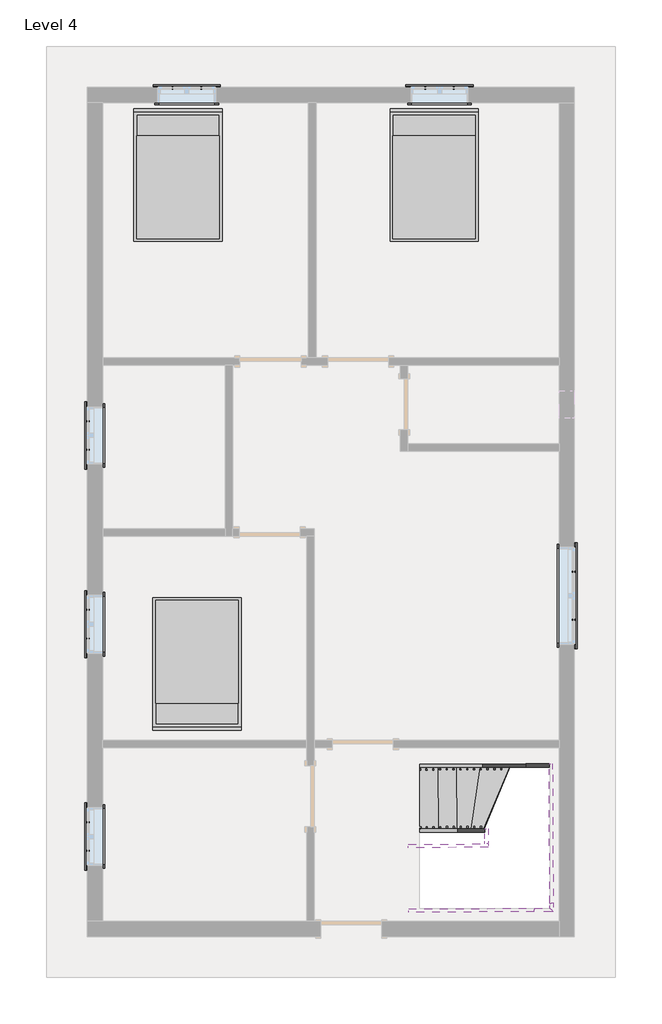
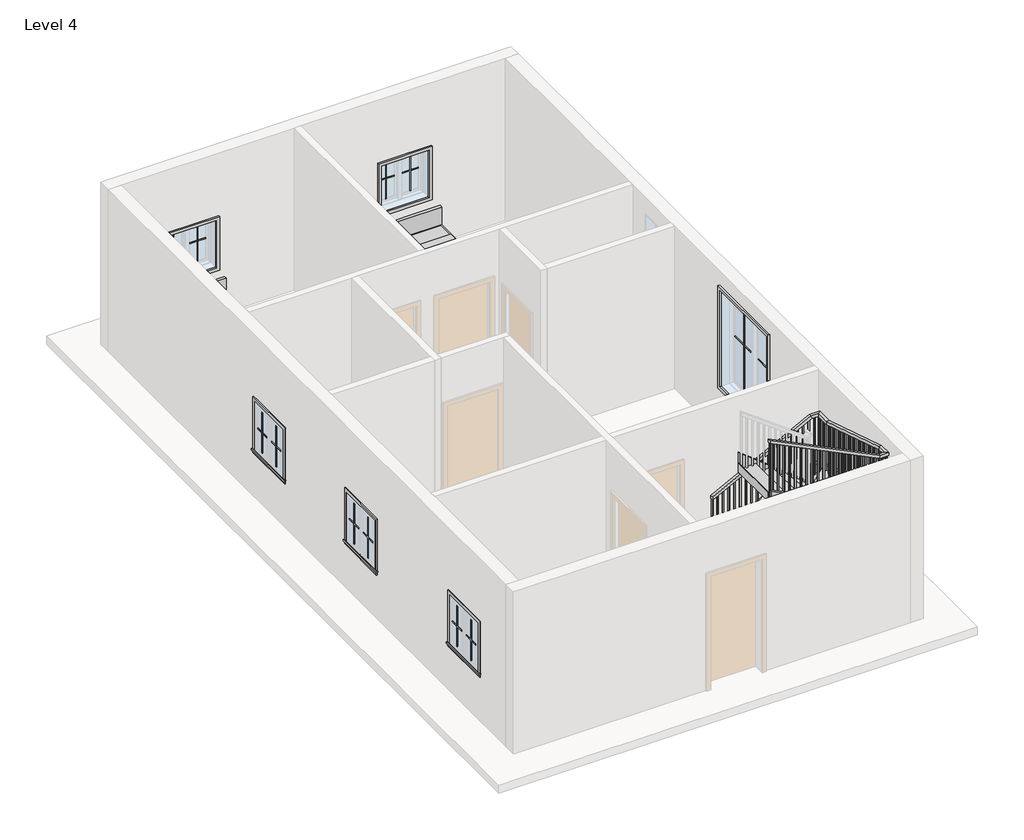
# One storey, part 2 of 2: 24 proxies, 9 members, 3 furniture elements, 1 railing, 1 stair flight.
"""IFC4 building model written with IfcOpenShell, lengths in millimetres."""

from ifc_helpers import new_model, si_unit, frame, origin, place, context, project, spatial, polyline, outline, extrude, faceted_brep, transform, mapped, element, save
from components import muntin_pattern_2x2_muntin_pattern_2x2_b3fe6957, muntin_pattern_2x2_muntin_pattern_2x2_3e0ecaf2, muntin_pattern_2x2_muntin_pattern_2x2_bff912c5, muntin_pattern_2x2_muntin_pattern_2x2_c2194282, trim_window_exterior_flat_with_sill_41619996, trim_window_exterior_flat_with_sill_e04b3088, trim_window_interior_flat_picture_frame_51c85655, trim_window_interior_flat_picture_frame_2a7685fe, bed_17739_bed_17739_15c61121, stair_flight_0f4fe1b0

model = new_model("IFC4")

# Units and contexts
model_context = context("Model", 3, world=origin())
ifc_project = project(units=[si_unit("LENGTHUNIT", "METRE", prefix="MILLI")], contexts=[model_context])

# Site, building, storey
site = spatial("IfcSite", under=ifc_project)
building = spatial("IfcBuilding", under=site)
storey = spatial("IfcBuildingStorey", under=building, Name="Level 4", Elevation=6400.8)

# Proxies
placement = place(None, origin())
muntin_pattern_2x2_muntin_pattern_2x2_shape = muntin_pattern_2x2_muntin_pattern_2x2_b3fe6957(model_context)
element("IfcBuildingElementProxy", 1, Name="Muntin Pattern_2x2 : Muntin Pattern_2x2", ObjectType="Muntin Pattern_2x2 : Muntin Pattern_2x2", at=placement, inside=storey, context=model_context, shape_type="MappedRepresentation", body=[
    mapped(muntin_pattern_2x2_muntin_pattern_2x2_shape, transform((-3622.2040084, 6872.3185985, 7385.05), x_axis=(1.0, 0.0, 0.0), y_axis=(0.0, 1.0, 0.0), z_axis=(0.0, 0.0, 1.0))),
])
element("IfcBuildingElementProxy", 2, Name="Muntin Pattern_2x2 : Muntin Pattern_2x2", ObjectType="Muntin Pattern_2x2 : Muntin Pattern_2x2", at=placement, inside=storey, context=model_context, shape_type="MappedRepresentation", body=[
    mapped(muntin_pattern_2x2_muntin_pattern_2x2_shape, transform((152.8709916, 6872.3185985, 7385.05), x_axis=(1.0, 0.0, 0.0), y_axis=(0.0, 1.0, 0.0), z_axis=(0.0, 0.0, 1.0))),
])
element("IfcBuildingElementProxy", 3, Name="Muntin Pattern_2x2 : Muntin Pattern_2x2", ObjectType="Muntin Pattern_2x2 : Muntin Pattern_2x2", at=placement, inside=storey, context=model_context, shape_type="MappedRepresentation", body=[
    mapped(muntin_pattern_2x2_muntin_pattern_2x2_shape, transform((-4884.2665084, 1466.8810985, 7385.05), x_axis=(0.0, 1.0, 0.0), y_axis=(-1.0, 0.0, 0.0), z_axis=(0.0, 0.0, 1.0))),
])
element("IfcBuildingElementProxy", 4, Name="Muntin Pattern_2x2 : Muntin Pattern_2x2", ObjectType="Muntin Pattern_2x2 : Muntin Pattern_2x2", at=placement, inside=storey, context=model_context, shape_type="MappedRepresentation", body=[
    mapped(muntin_pattern_2x2_muntin_pattern_2x2_shape, transform((-4884.2665084, -1352.5189015, 7385.05), x_axis=(0.0, 1.0, 0.0), y_axis=(-1.0, 0.0, 0.0), z_axis=(0.0, 0.0, 1.0))),
])
element("IfcBuildingElementProxy", 5, Name="Muntin Pattern_2x2 : Muntin Pattern_2x2", ObjectType="Muntin Pattern_2x2 : Muntin Pattern_2x2", at=placement, inside=storey, context=model_context, shape_type="MappedRepresentation", body=[
    mapped(muntin_pattern_2x2_muntin_pattern_2x2_shape, transform((-4884.2665084, -4524.3439015, 7385.05), x_axis=(0.0, 1.0, 0.0), y_axis=(-1.0, 0.0, 0.0), z_axis=(0.0, 0.0, 1.0))),
])
muntin_pattern_2x2_muntin_pattern_2x2_2_shape = muntin_pattern_2x2_muntin_pattern_2x2_3e0ecaf2(model_context)
element("IfcBuildingElementProxy", 6, Name="Muntin Pattern_2x2 : Muntin Pattern_2x2", ObjectType="Muntin Pattern_2x2 : Muntin Pattern_2x2", at=placement, inside=storey, context=model_context, shape_type="MappedRepresentation", body=[
    mapped(muntin_pattern_2x2_muntin_pattern_2x2_2_shape, transform((-3193.5790084, 6872.3185985, 7385.05), x_axis=(-1.0, 0.0, 0.0), y_axis=(0.0, -1.0, 0.0), z_axis=(0.0, 0.0, 1.0))),
])
element("IfcBuildingElementProxy", 7, Name="Muntin Pattern_2x2 : Muntin Pattern_2x2", ObjectType="Muntin Pattern_2x2 : Muntin Pattern_2x2", at=placement, inside=storey, context=model_context, shape_type="MappedRepresentation", body=[
    mapped(muntin_pattern_2x2_muntin_pattern_2x2_2_shape, transform((581.4959916, 6872.3185985, 7385.05), x_axis=(-1.0, 0.0, 0.0), y_axis=(0.0, -1.0, 0.0), z_axis=(0.0, 0.0, 1.0))),
])
element("IfcBuildingElementProxy", 8, Name="Muntin Pattern_2x2 : Muntin Pattern_2x2", ObjectType="Muntin Pattern_2x2 : Muntin Pattern_2x2", at=placement, inside=storey, context=model_context, shape_type="MappedRepresentation", body=[
    mapped(muntin_pattern_2x2_muntin_pattern_2x2_2_shape, transform((-4884.2665084, 1895.5060985, 7385.05), x_axis=(0.0, -1.0, 0.0), y_axis=(1.0, 0.0, 0.0), z_axis=(0.0, 0.0, 1.0))),
])
element("IfcBuildingElementProxy", 9, Name="Muntin Pattern_2x2 : Muntin Pattern_2x2", ObjectType="Muntin Pattern_2x2 : Muntin Pattern_2x2", at=placement, inside=storey, context=model_context, shape_type="MappedRepresentation", body=[
    mapped(muntin_pattern_2x2_muntin_pattern_2x2_2_shape, transform((-4884.2665084, -923.8939015, 7385.05), x_axis=(0.0, -1.0, 0.0), y_axis=(1.0, 0.0, 0.0), z_axis=(0.0, 0.0, 1.0))),
])
element("IfcBuildingElementProxy", 10, Name="Muntin Pattern_2x2 : Muntin Pattern_2x2", ObjectType="Muntin Pattern_2x2 : Muntin Pattern_2x2", at=placement, inside=storey, context=model_context, shape_type="MappedRepresentation", body=[
    mapped(muntin_pattern_2x2_muntin_pattern_2x2_2_shape, transform((-4884.2665084, -4095.7189015, 7385.05), x_axis=(0.0, -1.0, 0.0), y_axis=(1.0, 0.0, 0.0), z_axis=(0.0, 0.0, 1.0))),
])
muntin_pattern_2x2_muntin_pattern_2x2_3_shape = muntin_pattern_2x2_muntin_pattern_2x2_bff912c5(model_context)
element("IfcBuildingElementProxy", 11, Name="Muntin Pattern_2x2 : Muntin Pattern_2x2", ObjectType="Muntin Pattern_2x2 : Muntin Pattern_2x2", at=placement, inside=storey, context=model_context, shape_type="MappedRepresentation", body=[
    mapped(muntin_pattern_2x2_muntin_pattern_2x2_3_shape, transform((2373.7834916, -352.3939015, 7385.05), x_axis=(0.0, -1.0, 0.0), y_axis=(1.0, 0.0, 0.0), z_axis=(0.0, 0.0, 1.0))),
])
muntin_pattern_2x2_muntin_pattern_2x2_4_shape = muntin_pattern_2x2_muntin_pattern_2x2_c2194282(model_context)
element("IfcBuildingElementProxy", 12, Name="Muntin Pattern_2x2 : Muntin Pattern_2x2", ObjectType="Muntin Pattern_2x2 : Muntin Pattern_2x2", at=placement, inside=storey, context=model_context, shape_type="MappedRepresentation", body=[
    mapped(muntin_pattern_2x2_muntin_pattern_2x2_4_shape, transform((2373.7834916, -1073.1189015, 7385.05), x_axis=(0.0, 1.0, 0.0), y_axis=(-1.0, 0.0, 0.0), z_axis=(0.0, 0.0, 1.0))),
])
trim_window_exterior_flat_with_sill_shape = trim_window_exterior_flat_with_sill_41619996(model_context)
element("IfcBuildingElementProxy", 13, Name="Trim-Window-Exterior-Flat : with Sill", ObjectType="Trim-Window-Exterior-Flat : with Sill", at=placement, inside=storey, context=model_context, shape_type="MappedRepresentation", body=[
    mapped(trim_window_exterior_flat_with_sill_shape, transform((-3407.8915084, 6881.8435985, 8229.6), x_axis=(-1.0, 0.0, 0.0), y_axis=(0.0, 0.0, 1.0), z_axis=(0.0, 1.0, 0.0))),
])
element("IfcBuildingElementProxy", 14, Name="Trim-Window-Exterior-Flat : with Sill", ObjectType="Trim-Window-Exterior-Flat : with Sill", at=placement, inside=storey, context=model_context, shape_type="MappedRepresentation", body=[
    mapped(trim_window_exterior_flat_with_sill_shape, transform((367.1834916, 6881.8435985, 8229.6), x_axis=(-1.0, 0.0, 0.0), y_axis=(0.0, 0.0, 1.0), z_axis=(0.0, 1.0, 0.0))),
])
element("IfcBuildingElementProxy", 15, Name="Trim-Window-Exterior-Flat : with Sill", ObjectType="Trim-Window-Exterior-Flat : with Sill", at=placement, inside=storey, context=model_context, shape_type="MappedRepresentation", body=[
    mapped(trim_window_exterior_flat_with_sill_shape, transform((-4893.7915084, 1681.1935985, 8229.6), x_axis=(0.0, -1.0, 0.0), y_axis=(0.0, 0.0, 1.0), z_axis=(-1.0, 0.0, 0.0))),
])
element("IfcBuildingElementProxy", 16, Name="Trim-Window-Exterior-Flat : with Sill", ObjectType="Trim-Window-Exterior-Flat : with Sill", at=placement, inside=storey, context=model_context, shape_type="MappedRepresentation", body=[
    mapped(trim_window_exterior_flat_with_sill_shape, transform((-4893.7915084, -1138.2064015, 8229.6), x_axis=(0.0, -1.0, 0.0), y_axis=(0.0, 0.0, 1.0), z_axis=(-1.0, 0.0, 0.0))),
])
element("IfcBuildingElementProxy", 17, Name="Trim-Window-Exterior-Flat : with Sill", ObjectType="Trim-Window-Exterior-Flat : with Sill", at=placement, inside=storey, context=model_context, shape_type="MappedRepresentation", body=[
    mapped(trim_window_exterior_flat_with_sill_shape, transform((-4893.7915084, -4310.0314015, 8229.6), x_axis=(0.0, -1.0, 0.0), y_axis=(0.0, 0.0, 1.0), z_axis=(-1.0, 0.0, 0.0))),
])
trim_window_exterior_flat_with_sill_2_shape = trim_window_exterior_flat_with_sill_e04b3088(model_context)
element("IfcBuildingElementProxy", 18, Name="Trim-Window-Exterior-Flat : with Sill", ObjectType="Trim-Window-Exterior-Flat : with Sill", at=placement, inside=storey, context=model_context, shape_type="MappedRepresentation", body=[
    mapped(trim_window_exterior_flat_with_sill_2_shape, transform((2383.3084916, -712.7564015, 9144.0), x_axis=(0.0, 1.0, 0.0), y_axis=(0.0, 0.0, 1.0), z_axis=(1.0, 0.0, 0.0))),
])
trim_window_interior_flat_picture_frame_shape = trim_window_interior_flat_picture_frame_51c85655(model_context)
element("IfcBuildingElementProxy", 19, Name="Trim-Window-Interior-Flat : Picture Frame", ObjectType="Trim-Window-Interior-Flat : Picture Frame", at=placement, inside=storey, context=model_context, shape_type="MappedRepresentation", body=[
    mapped(trim_window_interior_flat_picture_frame_shape, transform((-3407.8915084, 6653.2435985, 8229.6), x_axis=(1.0, 0.0, 0.0), y_axis=(0.0, 0.0, 1.0), z_axis=(0.0, -1.0, 0.0))),
])
element("IfcBuildingElementProxy", 20, Name="Trim-Window-Interior-Flat : Picture Frame", ObjectType="Trim-Window-Interior-Flat : Picture Frame", at=placement, inside=storey, context=model_context, shape_type="MappedRepresentation", body=[
    mapped(trim_window_interior_flat_picture_frame_shape, transform((367.1834916, 6653.2435985, 8229.6), x_axis=(1.0, 0.0, 0.0), y_axis=(0.0, 0.0, 1.0), z_axis=(0.0, -1.0, 0.0))),
])
element("IfcBuildingElementProxy", 21, Name="Trim-Window-Interior-Flat : Picture Frame", ObjectType="Trim-Window-Interior-Flat : Picture Frame", at=placement, inside=storey, context=model_context, shape_type="MappedRepresentation", body=[
    mapped(trim_window_interior_flat_picture_frame_shape, transform((-4665.1915084, 1681.1935985, 8229.6), x_axis=(0.0, 1.0, 0.0), y_axis=(0.0, 0.0, 1.0), z_axis=(1.0, 0.0, 0.0))),
])
element("IfcBuildingElementProxy", 22, Name="Trim-Window-Interior-Flat : Picture Frame", ObjectType="Trim-Window-Interior-Flat : Picture Frame", at=placement, inside=storey, context=model_context, shape_type="MappedRepresentation", body=[
    mapped(trim_window_interior_flat_picture_frame_shape, transform((-4665.1915084, -1138.2064015, 8229.6), x_axis=(0.0, 1.0, 0.0), y_axis=(0.0, 0.0, 1.0), z_axis=(1.0, 0.0, 0.0))),
])
element("IfcBuildingElementProxy", 23, Name="Trim-Window-Interior-Flat : Picture Frame", ObjectType="Trim-Window-Interior-Flat : Picture Frame", at=placement, inside=storey, context=model_context, shape_type="MappedRepresentation", body=[
    mapped(trim_window_interior_flat_picture_frame_shape, transform((-4665.1915084, -4310.0314015, 8229.6), x_axis=(0.0, 1.0, 0.0), y_axis=(0.0, 0.0, 1.0), z_axis=(1.0, 0.0, 0.0))),
])
trim_window_interior_flat_picture_frame_2_shape = trim_window_interior_flat_picture_frame_2a7685fe(model_context)
element("IfcBuildingElementProxy", 24, Name="Trim-Window-Interior-Flat : Picture Frame", ObjectType="Trim-Window-Interior-Flat : Picture Frame", at=placement, inside=storey, context=model_context, shape_type="MappedRepresentation", body=[
    mapped(trim_window_interior_flat_picture_frame_2_shape, transform((2154.7084916, -712.7564015, 9144.0), x_axis=(0.0, -1.0, 0.0), y_axis=(0.0, 0.0, 1.0), z_axis=(-1.0, 0.0, 0.0))),
])

# Furniture
bed_17739_bed_17739_shape = bed_17739_bed_17739_15c61121(model_context)
element("IfcFurniture", 25, ObjectType="Bed_17739 : Bed_17739", at=placement, inside=storey, context=model_context, shape_type="MappedRepresentation", body=[
    mapped(bed_17739_bed_17739_shape, transform((-3541.2415084, 5548.3435985, 6400.8), x_axis=(1.0, 0.0, 0.0), y_axis=(0.0, 1.0, 0.0), z_axis=(0.0, 0.0, 1.0))),
])
element("IfcFurniture", 26, ObjectType="Bed_17739 : Bed_17739", at=placement, inside=storey, context=model_context, shape_type="MappedRepresentation", body=[
    mapped(bed_17739_bed_17739_shape, transform((287.8084916, 5548.3435985, 6400.8), x_axis=(1.0, 0.0, 0.0), y_axis=(0.0, 1.0, 0.0), z_axis=(0.0, 0.0, 1.0))),
])
element("IfcFurniture", 27, ObjectType="Bed_17739 : Bed_17739", at=placement, inside=storey, context=model_context, shape_type="MappedRepresentation", body=[
    mapped(bed_17739_bed_17739_shape, transform((-3255.4915084, -1709.7064015, 6400.8), x_axis=(-1.0, 0.0, 0.0), y_axis=(0.0, -1.0, 0.0), z_axis=(0.0, 0.0, 1.0))),
])

# Members
element("IfcMember", 28, ObjectType="Stringer - 2\" Width", at=placement, inside=storey, context=model_context, shape_type="SweptSolid", body=[
    extrude(outline(polyline([(149.3129896, -304.8), (0.0, 0.0), (1768.8429208, 0.0), (1918.1559104, -304.8000001), (149.3129896, -304.8)])), frame((68.8012135, -3282.7418259, 6804.1997735), z_axis=(-0.005162073969671357, 0.9999866764074068, 0.0), x_axis=(0.8980237466183221, 0.0046357267711000134, 0.43992256198892044)), (0.0, 0.0, 1.0), 50.8),
])
element("IfcMember", 29, ObjectType="Stringer - 2\" Width", at=placement, inside=storey, context=model_context, shape_type="SweptSolid", body=[
    extrude(outline(polyline([(1657.2641604, -3274.5419534), (1657.0019271, -3223.7426303), (2003.5241973, -3221.9538329), (2003.7864306, -3272.753156), (1657.2641604, -3274.5419534)])), frame((0.0, 0.0, 7582.353683), z_axis=(0.0, 0.0, 1.0), x_axis=(1.0, 0.0, 0.0)), (0.0, 0.0, 1.0), 339.4074379),
])
element("IfcMember", 30, ObjectType="Stringer - 2\" Width", at=placement, inside=storey, context=model_context, shape_type="SweptSolid", body=[
    extrude(outline(polyline([(47.2049979, -324.2228076), (-38.2916769, -48.0839082), (117.0107078, 0.0), (2125.7436964, 0.0), (2226.1278582, -324.2228076), (47.2049979, -324.2228076)])), frame((2003.7864306, -3272.753156, 7582.353683), z_axis=(0.9999866764074068, 0.005162073969671768, 0.0), x_axis=(0.004931129753271623, -0.9552486233011703, 0.2957629991066754)), (0.0, 0.0, 1.0), 50.8),
])
element("IfcMember", 31, ObjectType="Stringer - 2\" Width", at=placement, inside=storey, context=model_context, shape_type="SweptSolid", body=[
    extrude(outline(polyline([(2014.2687486, -5303.3668955), (2065.0680718, -5303.1046621), (2065.7306715, -5431.462157), (2014.669115, -5380.9250672), (2014.2687486, -5303.3668955)])), frame((0.0, 0.0, 8221.0291102), z_axis=(0.0, 0.0, 1.0), x_axis=(1.0, 0.0, 0.0)), (0.0, 0.0, 1.0), 319.0749838),
])
element("IfcMember", 32, ObjectType="Stringer - 2\" Width", at=placement, inside=storey, context=model_context, shape_type="SweptSolid", body=[
    extrude(outline(polyline([(2014.669115, -5380.9250672), (2065.7306715, -5431.462157), (1782.4368375, -5432.9245602), (1782.1746041, -5382.1252371), (2014.669115, -5380.9250672)])), frame((0.0, 0.0, 8221.0291102), z_axis=(0.0, 0.0, 1.0), x_axis=(1.0, 0.0, 0.0)), (0.0, 0.0, 1.0), 319.0749838),
])
element("IfcMember", 33, ObjectType="Stringer - 2\" Width", at=placement, inside=storey, context=model_context, shape_type="SweptSolid", body=[
    extrude(outline(polyline([(286.8047106, -304.8), (0.0, 0.0), (1331.6484515, 0.0), (1618.4531621, -304.8), (286.8047106, -304.8)])), frame((73.7836473, -4247.928966, 6647.3616111), z_axis=(-0.005162073969671482, 0.9999866764074068, 0.0), x_axis=(0.7282688430294204, 0.0037594277266083504, 0.6852812261953175)), (0.0, 0.0, 1.0), 50.8),
])
element("IfcMember", 34, ObjectType="Stringer - 2\" Width", at=placement, inside=storey, context=model_context, shape_type="SweptSolid", body=[
    extrude(outline(polyline([(660.780085, -304.8), (110.7389009, -51.080863), (134.3011229, 0.0), (545.7678218, 0.0), (1125.9670058, -267.6302075), (1108.8215849, -304.8), (660.780085, -304.8)])), frame((1043.319491, -4192.1234067, 7485.7637993), z_axis=(0.9999866764074068, 0.005162073969671282, 0.0), x_axis=(0.002162183372020065, -0.4188538515087163, 0.90805108669027)), (0.0, 0.0, 1.0), 50.8),
])
element("IfcMember", 35, ObjectType="Stringer - 2\" Width", at=placement, inside=storey, context=model_context, shape_type="SweptSolid", body=[
    extrude(outline(polyline([(-239.6623642, -304.8), (0.0, 0.0), (1521.9461582, 0.0), (1282.2837939, -304.8), (-239.6623642, -304.8)])), frame((1095.5610976, -4471.2574507, 8620.2987993), z_axis=(-0.005162073969672184, 0.9999866764074068, 0.0), x_axis=(-0.7860864868637559, -0.0040578906574323574, 0.6181032023000775)), (0.0, 0.0, 1.0), 50.8),
])
element("IfcMember", 36, ObjectType="Stringer - 2\" Width", at=placement, inside=storey, context=model_context, shape_type="SweptSolid", body=[
    extrude(outline(polyline([(-137.2719745, -288.0368905), (0.0, 0.0), (2080.7002403, 0.0), (1943.4282658, -288.0368905), (-137.2719745, -288.0368905)])), frame((1782.4368375, -5432.9245602, 8540.104094), z_axis=(-0.005162073969672376, 0.9999866764074068, 0.0), x_axis=(-0.9027127399072911, -0.004659932023802854, 0.43021854242071556)), (0.0, 0.0, 1.0), 50.8),
])

# Railing
element("IfcRailing", 37, ObjectType="Handrail - Rectangular", at=placement, inside=storey, context=model_context, shape_type="SolidModel", body=[
    faceted_brep([(68.8012135, -3282.7418259, 7992.5333333), (68.8012135, -3282.7418259, 7935.4032367), (69.0634468, -3333.5411491, 7935.4032367), (69.0634468, -3333.5411491, 7992.5333333), (1818.9474855, -3273.707321, 8893.0523232), (1831.2499413, -3273.643814, 8842.2523232), (1831.5121746, -3324.4431372, 8842.2523232), (1819.2097188, -3324.5066442, 8893.0523232), (2003.7864306, -3272.753156, 8893.0523232), (2003.7864306, -3272.753156, 8842.2523232), (1953.2493408, -3323.8147125, 8842.2523232), (1953.2493408, -3323.8147125, 8893.0523232), (2005.285328, -3563.1165554, 8893.0523232), (2005.3249947, -3570.8007251, 8842.2523232), (1954.5256716, -3571.0629585, 8842.2523232), (1954.4860048, -3563.3787887, 8893.0523232), (2013.5123671, -5156.842168, 9386.4998462), (2013.5520339, -5164.5263378, 9335.6998462), (1962.7527107, -5164.7885712, 9335.6998462), (1962.7130439, -5157.1044014, 9386.4998462), (2014.669115, -5380.9250672, 9386.4998462), (2014.669115, -5380.9250672, 9335.6998462), (1963.6075585, -5330.3879774, 9335.6998462), (1963.6075585, -5330.3879774, 9386.4998462), (1865.7077622, -5381.694027, 9386.4998462), (1853.7618085, -5381.7556937, 9335.6998462), (1853.4995752, -5330.9563705, 9335.6998462), (1865.4455288, -5330.8947038, 9386.4998462), (-96.1000106, -5391.8211588, 10363.2), (-96.362244, -5341.0218356, 10363.2), (-96.362244, -5341.0218356, 10306.4526208), (-96.1000106, -5391.8211588, 10306.4526208)], [[[0, 1, 2, 3]], [[1, 0, 4, 5]], [[2, 1, 5, 6]], [[3, 2, 6, 7]], [[0, 3, 7, 4]], [[5, 4, 8, 9]], [[6, 5, 9, 10]], [[7, 6, 10, 11]], [[4, 7, 11, 8]], [[9, 8, 12, 13]], [[10, 9, 13, 14]], [[11, 10, 14, 15]], [[8, 11, 15, 12]], [[13, 12, 16, 17]], [[14, 13, 17, 18]], [[15, 14, 18, 19]], [[12, 15, 19, 16]], [[17, 16, 20, 21]], [[18, 17, 21, 22]], [[19, 18, 22, 23]], [[16, 19, 23, 20]], [[21, 20, 24, 25]], [[22, 21, 25, 26]], [[23, 22, 26, 27]], [[20, 23, 27, 24]], [[28, 29, 30, 31]], [[25, 24, 28, 31]], [[26, 25, 31, 30]], [[27, 26, 30, 29]], [[24, 27, 29, 28]]]),
    extrude(outline(polyline([(223.8579732, 19.05), (1229.0021026, 19.05), (1229.0021026, 0.0), (233.3420268, 0.0), (223.8579732, 19.05)])), frame((-33.2605479, -5375.621561, 10508.4687693), z_axis=(-0.005162073969671937, 0.9999866764074068, 0.0), x_axis=(0.0, 0.0, -1.0)), (0.0, 0.0, 1.0), 19.05),
    extrude(outline(polyline([(223.8579732, 19.0499999), (1178.4204835, 19.0499999), (1178.4204835, 0.0), (233.3420268, 0.0), (223.8579732, 19.0499999)])), frame((68.3380984, -5375.0970942, 10457.8871502), z_axis=(-0.005162073969671937, 0.9999866764074068, 0.0), x_axis=(0.0, 0.0, -1.0)), (0.0, 0.0, 1.0), 19.05),
    extrude(outline(polyline([(223.8579732, 19.05), (1127.8388644, 19.05), (1127.8388644, 0.0), (233.3420268, 0.0), (223.8579732, 19.05)])), frame((169.9367448, -5374.5726275, 10407.3055311), z_axis=(-0.005162073969671937, 0.9999866764074068, 0.0), x_axis=(0.0, 0.0, -1.0)), (0.0, 0.0, 1.0), 19.05),
    extrude(outline(polyline([(223.8579732, 19.05), (1246.5905787, 19.05), (1246.5905787, 0.0), (233.3420268, 0.0), (223.8579732, 19.05)])), frame((271.5353911, -5374.0481608, 10356.723912), z_axis=(-0.005162073969671937, 0.9999866764074068, 0.0), x_axis=(0.0, 0.0, -1.0)), (0.0, 0.0, 1.0), 19.05),
    extrude(outline(polyline([(223.8579732, 19.05), (1196.0089596, 19.05), (1196.0089596, 0.0), (233.3420267, 0.0), (223.8579732, 19.05)])), frame((373.1340374, -5373.5236941, 10306.1422929), z_axis=(-0.005162073969671937, 0.9999866764074068, 0.0), x_axis=(0.0, 0.0, -1.0)), (0.0, 0.0, 1.0), 19.05),
    extrude(outline(polyline([(223.8579732, 19.05), (1314.7606738, 19.05), (1314.7606738, 0.0), (233.3420267, 0.0), (223.8579732, 19.05)])), frame((474.7326837, -5372.9992274, 10255.5606738), z_axis=(-0.005162073969671937, 0.9999866764074068, 0.0), x_axis=(0.0, 0.0, -1.0)), (0.0, 0.0, 1.0), 19.05),
    extrude(outline(polyline([(223.8579733, 19.05), (1264.1790548, 19.05), (1264.1790548, 0.0), (233.3420268, 0.0), (223.8579733, 19.05)])), frame((576.3313301, -5372.4747607, 10204.9790548), z_axis=(-0.005162073969671937, 0.9999866764074068, 0.0), x_axis=(0.0, 0.0, -1.0)), (0.0, 0.0, 1.0), 19.05),
    extrude(outline(polyline([(223.8579732, 19.05), (1213.5974357, 19.05), (1213.5974357, 0.0), (233.3420268, 0.0), (223.8579732, 19.05)])), frame((677.9299764, -5371.950294, 10154.3974357), z_axis=(-0.005162073969671937, 0.9999866764074068, 0.0), x_axis=(0.0, 0.0, -1.0)), (0.0, 0.0, 1.0), 19.05),
    extrude(outline(polyline([(223.8579732, 19.05), (1163.0158166, 19.05), (1163.0158166, 0.0), (233.3420268, 0.0), (223.8579732, 19.05)])), frame((779.5286227, -5371.4258272, 10103.8158166), z_axis=(-0.005162073969671937, 0.9999866764074068, 0.0), x_axis=(0.0, 0.0, -1.0)), (0.0, 0.0, 1.0), 19.05),
    extrude(outline(polyline([(223.8579732, 19.05), (1281.7675308, 19.05), (1281.7675308, 0.0), (233.3420268, 0.0), (223.8579732, 19.05)])), frame((881.127269, -5370.9013605, 10053.2341975), z_axis=(-0.005162073969671937, 0.9999866764074068, 0.0), x_axis=(0.0, 0.0, -1.0)), (0.0, 0.0, 1.0), 19.05),
    extrude(outline(polyline([(223.8579732, 19.0499999), (1231.1859117, 19.0499999), (1231.1859117, 0.0), (233.3420268, 0.0), (223.8579732, 19.0499999)])), frame((982.7259153, -5370.3768938, 10002.6525784), z_axis=(-0.005162073969671937, 0.9999866764074068, 0.0), x_axis=(0.0, 0.0, -1.0)), (0.0, 0.0, 1.0), 19.05),
    extrude(outline(polyline([(223.8579732, 19.05), (1180.6042926, 19.05), (1180.6042926, 0.0), (233.3420268, 0.0), (223.8579732, 19.05)])), frame((1084.3245617, -5369.8524271, 9952.0709593), z_axis=(-0.005162073969671937, 0.9999866764074068, 0.0), x_axis=(0.0, 0.0, -1.0)), (0.0, 0.0, 1.0), 19.05),
    extrude(outline(polyline([(223.8579732, 19.05), (1299.3560069, 19.05), (1299.3560069, 0.0), (233.3420268, 0.0), (223.8579732, 19.05)])), frame((1185.923208, -5369.3279604, 9901.4893402), z_axis=(-0.005162073969671937, 0.9999866764074068, 0.0), x_axis=(0.0, 0.0, -1.0)), (0.0, 0.0, 1.0), 19.05),
    extrude(outline(polyline([(223.8579732, 19.05), (1248.7743878, 19.05), (1248.7743878, 0.0), (233.3420268, 0.0), (223.8579732, 19.05)])), frame((1287.5218543, -5368.8034937, 9850.9077211), z_axis=(-0.005162073969671937, 0.9999866764074068, 0.0), x_axis=(0.0, 0.0, -1.0)), (0.0, 0.0, 1.0), 19.05),
    extrude(outline(polyline([(223.8579732, 19.0499999), (1198.1927687, 19.0499999), (1198.1927687, 0.0), (233.3420268, 0.0), (223.8579732, 19.0499999)])), frame((1389.1205006, -5368.2790269, 9800.326102), z_axis=(-0.005162073969671937, 0.9999866764074068, 0.0), x_axis=(0.0, 0.0, -1.0)), (0.0, 0.0, 1.0), 19.05),
    extrude(outline(polyline([(223.8579732, 19.05), (1147.6111496, 19.05), (1147.6111496, 0.0), (233.3420268, 0.0), (223.8579732, 19.05)])), frame((1490.719147, -5367.7545602, 9749.7444829), z_axis=(-0.005162073969671937, 0.9999866764074068, 0.0), x_axis=(0.0, 0.0, -1.0)), (0.0, 0.0, 1.0), 19.05),
    extrude(outline(polyline([(223.8579732, 19.05), (1097.0295305, 19.05), (1097.0295305, 0.0), (233.3420267, 0.0), (223.8579732, 19.05)])), frame((1592.3177933, -5367.2300935, 9699.1628638), z_axis=(-0.005162073969671937, 0.9999866764074068, 0.0), x_axis=(0.0, 0.0, -1.0)), (0.0, 0.0, 1.0), 19.05),
    extrude(outline(polyline([(223.8579733, 19.05), (1215.7812448, 19.05), (1215.7812448, 0.0), (233.3420268, 0.0), (223.8579733, 19.05)])), frame((1693.9164396, -5366.7056268, 9648.5812448), z_axis=(-0.005162073969671937, 0.9999866764074068, 0.0), x_axis=(0.0, 0.0, -1.0)), (0.0, 0.0, 1.0), 19.05),
    extrude(outline(polyline([(223.8579733, 19.05), (1165.1996257, 19.05), (1165.1996257, 0.0), (233.3420268, 0.0), (223.8579733, 19.05)])), frame((1795.5150859, -5366.1811601, 9597.9996257), z_axis=(-0.005162073969671937, 0.9999866764074068, 0.0), x_axis=(0.0, 0.0, -1.0)), (0.0, 0.0, 1.0), 19.05),
    extrude(outline(polyline([(1897.1137323, -5365.6566934), (1878.0639861, -5365.7550309), (1877.9656486, -5346.7052847), (1897.0153947, -5346.6069472), (1897.1137323, -5365.6566934)])), frame((0.0, 0.0, 8432.8), z_axis=(0.0, 0.0, 1.0), x_axis=(1.0, 0.0, 0.0)), (0.0, 0.0, 1.0), 902.8998462),
    extrude(outline(polyline([(1998.4829244, -5320.6828189), (1998.5812619, -5339.7325651), (1979.5315157, -5339.8309026), (1979.4331782, -5320.7811564), (1998.4829244, -5320.6828189)])), frame((0.0, 0.0, 8432.8), z_axis=(0.0, 0.0, 1.0), x_axis=(1.0, 0.0, 0.0)), (0.0, 0.0, 1.0), 902.8998462),
    extrude(outline(polyline([(1997.9584577, -5219.0841726), (1998.0567952, -5238.1339187), (1979.007049, -5238.2322563), (1978.9087115, -5219.1825101), (1997.9584577, -5219.0841726)])), frame((0.0, 0.0, 8432.8), z_axis=(0.0, 0.0, 1.0), x_axis=(1.0, 0.0, 0.0)), (0.0, 0.0, 1.0), 902.8998462),
    extrude(outline(polyline([(231.5490805, 19.05), (1119.8588311, 19.05), (1119.8588311, 0.0), (225.6509196, 0.0), (231.5490805, 19.05)])), frame((1978.4825823, -5136.6336099, 9552.6588311), z_axis=(0.9999866764074068, 0.005162073969671697, 0.0), x_axis=(0.0, 0.0, -1.0)), (0.0, 0.0, 1.0), 19.05),
    extrude(outline(polyline([(231.5490804, 19.05), (1088.401973, 19.05), (1088.401973, 0.0), (225.6509195, 0.0), (231.5490804, 19.05)])), frame((1977.9581156, -5035.0349636, 9521.201973), z_axis=(0.9999866764074068, 0.005162073969671697, 0.0), x_axis=(0.0, 0.0, -1.0)), (0.0, 0.0, 1.0), 19.05),
    extrude(outline(polyline([(231.5490805, 19.05), (1226.2784483, 19.05), (1226.2784483, 0.0), (225.6509196, 0.0), (231.5490805, 19.05)])), frame((1977.4336488, -4933.4363173, 9489.745115), z_axis=(0.9999866764074068, 0.005162073969671697, 0.0), x_axis=(0.0, 0.0, -1.0)), (0.0, 0.0, 1.0), 19.05),
    extrude(outline(polyline([(231.5490804, 19.05), (1194.8215902, 19.05), (1194.8215902, 0.0), (225.6509195, 0.0), (231.5490804, 19.05)])), frame((1976.9091821, -4831.837671, 9458.2882569), z_axis=(0.9999866764074068, 0.005162073969671697, 0.0), x_axis=(0.0, 0.0, -1.0)), (0.0, 0.0, 1.0), 19.05),
    extrude(outline(polyline([(231.5490805, 19.0499999), (1163.3647322, 19.0499999), (1163.3647322, 0.0), (225.6509196, 0.0), (231.5490805, 19.0499999)])), frame((1976.3847154, -4730.2390246, 9426.8313989), z_axis=(0.9999866764074068, 0.005162073969671697, 0.0), x_axis=(0.0, 0.0, -1.0)), (0.0, 0.0, 1.0), 19.05),
    extrude(outline(polyline([(231.5490804, 19.05), (1131.9078741, 19.05), (1131.9078741, 0.0), (225.6509195, 0.0), (231.5490804, 19.05)])), frame((1975.8602487, -4628.6403783, 9395.3745408), z_axis=(0.9999866764074068, 0.005162073969671697, 0.0), x_axis=(0.0, 0.0, -1.0)), (0.0, 0.0, 1.0), 19.05),
    extrude(outline(polyline([(231.5490805, 19.05), (1100.4510161, 19.05), (1100.4510161, 0.0), (225.6509196, 0.0), (231.5490805, 19.05)])), frame((1975.335782, -4527.041732, 9363.9176828), z_axis=(0.9999866764074068, 0.005162073969671697, 0.0), x_axis=(0.0, 0.0, -1.0)), (0.0, 0.0, 1.0), 19.05),
    extrude(outline(polyline([(231.5490804, 19.05), (1238.3274914, 19.05), (1238.3274914, 0.0), (225.6509195, 0.0), (231.5490804, 19.05)])), frame((1974.8113153, -4425.4430857, 9332.4608247), z_axis=(0.9999866764074068, 0.005162073969671697, 0.0), x_axis=(0.0, 0.0, -1.0)), (0.0, 0.0, 1.0), 19.05),
    extrude(outline(polyline([(231.5490805, 19.05), (1206.8706334, 19.05), (1206.8706334, 0.0), (225.6509196, 0.0), (231.5490805, 19.05)])), frame((1974.2868486, -4323.8444394, 9301.0039667), z_axis=(0.9999866764074068, 0.005162073969671697, 0.0), x_axis=(0.0, 0.0, -1.0)), (0.0, 0.0, 1.0), 19.05),
    extrude(outline(polyline([(231.5490804, 19.05), (1175.4137753, 19.05), (1175.4137753, 0.0), (225.6509195, 0.0), (231.5490804, 19.05)])), frame((1973.7623818, -4222.245793, 9269.5471086), z_axis=(0.9999866764074068, 0.005162073969671697, 0.0), x_axis=(0.0, 0.0, -1.0)), (0.0, 0.0, 1.0), 19.05),
    extrude(outline(polyline([(231.5490804, 19.05), (1143.9569173, 19.05), (1143.9569173, 0.0), (225.6509196, 0.0), (231.5490804, 19.05)])), frame((1973.2379151, -4120.6471467, 9238.0902506), z_axis=(0.9999866764074068, 0.005162073969671697, 0.0), x_axis=(0.0, 0.0, -1.0)), (0.0, 0.0, 1.0), 19.05),
    extrude(outline(polyline([(231.5490805, 19.05), (1281.8333926, 19.05), (1281.8333926, 0.0), (225.6509196, 0.0), (231.5490805, 19.05)])), frame((1972.7134484, -4019.0485004, 9206.6333926), z_axis=(0.9999866764074068, 0.005162073969671697, 0.0), x_axis=(0.0, 0.0, -1.0)), (0.0, 0.0, 1.0), 19.05),
    extrude(outline(polyline([(231.5490804, 19.05), (1250.3765345, 19.05), (1250.3765345, 0.0), (225.6509196, 0.0), (231.5490804, 19.05)])), frame((1972.1889817, -3917.4498541, 9175.1765345), z_axis=(0.9999866764074068, 0.005162073969671697, 0.0), x_axis=(0.0, 0.0, -1.0)), (0.0, 0.0, 1.0), 19.05),
    extrude(outline(polyline([(231.5490805, 19.0499999), (1218.9196765, 19.0499999), (1218.9196765, 0.0), (225.6509196, 0.0), (231.5490805, 19.0499999)])), frame((1971.664515, -3815.8512077, 9143.7196765), z_axis=(0.9999866764074068, 0.005162073969671697, 0.0), x_axis=(0.0, 0.0, -1.0)), (0.0, 0.0, 1.0), 19.05),
    extrude(outline(polyline([(231.5490804, 19.05), (1187.4628184, 19.05), (1187.4628184, 0.0), (225.6509195, 0.0), (231.5490804, 19.05)])), frame((1971.1400483, -3714.2525614, 9112.2628184), z_axis=(0.9999866764074068, 0.005162073969671697, 0.0), x_axis=(0.0, 0.0, -1.0)), (0.0, 0.0, 1.0), 19.05),
    extrude(outline(polyline([(231.5490805, 19.05), (1156.0059604, 19.05), (1156.0059604, 0.0), (225.6509196, 0.0), (231.5490805, 19.05)])), frame((1970.6155816, -3612.6539151, 9080.8059604), z_axis=(0.9999866764074068, 0.005162073969671697, 0.0), x_axis=(0.0, 0.0, -1.0)), (0.0, 0.0, 1.0), 19.05),
    extrude(outline(polyline([(1989.0425235, -3491.9071851), (1989.140861, -3510.9569313), (1970.0911148, -3511.0552688), (1969.9927773, -3492.0055226), (1989.0425235, -3491.9071851)])), frame((0.0, 0.0, 7924.8), z_axis=(0.0, 0.0, 1.0), x_axis=(1.0, 0.0, 0.0)), (0.0, 0.0, 1.0), 917.4523232),
    extrude(outline(polyline([(1988.5180568, -3390.3085387), (1988.6163943, -3409.3582849), (1969.5666481, -3409.4566224), (1969.4683106, -3390.4068763), (1988.5180568, -3390.3085387)])), frame((0.0, 0.0, 7755.4666667), z_axis=(0.0, 0.0, 1.0), x_axis=(1.0, 0.0, 0.0)), (0.0, 0.0, 1.0), 1086.7856565),
    extrude(outline(polyline([(1888.1339221, -3289.2253823), (1907.1836683, -3289.1270448), (1907.2820058, -3308.176791), (1888.2322596, -3308.2751285), (1888.1339221, -3289.2253823)])), frame((0.0, 0.0, 7755.4666667), z_axis=(0.0, 0.0, 1.0), x_axis=(1.0, 0.0, 0.0)), (0.0, 0.0, 1.0), 1086.7856565),
    extrude(outline(polyline([(233.5009213, 19.05), (1297.2369609, 19.05), (1297.2369609, 0.0), (223.6990787, 0.0), (233.5009213, 19.05)])), frame((1805.6833595, -3308.7012577, 9052.7036276), z_axis=(-0.005162073969671542, 0.9999866764074069, 0.0), x_axis=(0.0, 0.0, -1.0)), (0.0, 0.0, 1.0), 19.05),
    extrude(outline(polyline([(233.5009213, 19.05), (1244.9604673, 19.05), (1244.9604673, 0.0), (223.6990787, 0.0), (233.5009213, 19.05)])), frame((1704.0847132, -3309.2257244, 9000.427134), z_axis=(-0.005162073969671542, 0.9999866764074069, 0.0), x_axis=(0.0, 0.0, -1.0)), (0.0, 0.0, 1.0), 19.05),
    extrude(outline(polyline([(233.5009212, 19.05), (1192.6839737, 19.05), (1192.6839737, 0.0), (223.6990787, 0.0), (233.5009212, 19.05)])), frame((1602.4860668, -3309.7501911, 8948.1506404), z_axis=(-0.005162073969671542, 0.9999866764074069, 0.0), x_axis=(0.0, 0.0, -1.0)), (0.0, 0.0, 1.0), 19.05),
    extrude(outline(polyline([(233.5009212, 19.05), (1140.4074801, 19.05), (1140.4074801, 0.0), (223.6990787, 0.0), (233.5009212, 19.05)])), frame((1500.8874205, -3310.2746578, 8895.8741468), z_axis=(-0.005162073969671542, 0.9999866764074069, 0.0), x_axis=(0.0, 0.0, -1.0)), (0.0, 0.0, 1.0), 19.05),
    extrude(outline(polyline([(233.5009213, 19.05), (1088.1309866, 19.05), (1088.1309866, 0.0), (223.6990788, 0.0), (233.5009213, 19.05)])), frame((1399.2887742, -3310.7991245, 8843.5976533), z_axis=(-0.005162073969671542, 0.9999866764074069, 0.0), x_axis=(0.0, 0.0, -1.0)), (0.0, 0.0, 1.0), 19.05),
    extrude(outline(polyline([(233.5009213, 19.05), (1205.1878264, 19.05), (1205.1878264, 0.0), (223.6990788, 0.0), (233.5009213, 19.05)])), frame((1297.6901279, -3311.3235913, 8791.3211597), z_axis=(-0.005162073969671542, 0.9999866764074069, 0.0), x_axis=(0.0, 0.0, -1.0)), (0.0, 0.0, 1.0), 19.05),
    extrude(outline(polyline([(233.5009213, 19.0499999), (1152.9113328, 19.0499999), (1152.9113328, 0.0), (223.6990787, 0.0), (233.5009213, 19.0499999)])), frame((1196.0914815, -3311.848058, 8739.0446661), z_axis=(-0.005162073969671542, 0.9999866764074069, 0.0), x_axis=(0.0, 0.0, -1.0)), (0.0, 0.0, 1.0), 19.05),
    extrude(outline(polyline([(233.5009213, 19.05), (1100.6348392, 19.05), (1100.6348392, 0.0), (223.6990787, 0.0), (233.5009213, 19.05)])), frame((1094.4928352, -3312.3725247, 8686.7681725), z_axis=(-0.005162073969671542, 0.9999866764074069, 0.0), x_axis=(0.0, 0.0, -1.0)), (0.0, 0.0, 1.0), 19.05),
    extrude(outline(polyline([(233.5009213, 19.05), (1048.3583456, 19.05), (1048.3583456, 0.0), (223.6990787, 0.0), (233.5009213, 19.05)])), frame((992.8941889, -3312.8969914, 8634.4916789), z_axis=(-0.005162073969671542, 0.9999866764074069, 0.0), x_axis=(0.0, 0.0, -1.0)), (0.0, 0.0, 1.0), 19.05),
    extrude(outline(polyline([(233.5009212, 19.05), (1165.4151853, 19.05), (1165.4151853, 0.0), (223.6990787, 0.0), (233.5009212, 19.05)])), frame((891.2955426, -3313.4214581, 8582.2151853), z_axis=(-0.005162073969671542, 0.9999866764074069, 0.0), x_axis=(0.0, 0.0, -1.0)), (0.0, 0.0, 1.0), 19.05),
    extrude(outline(polyline([(233.5009213, 19.0499999), (1113.1386918, 19.0499999), (1113.1386918, 0.0), (223.6990788, 0.0), (233.5009213, 19.0499999)])), frame((789.6968962, -3313.9459248, 8529.9386918), z_axis=(-0.005162073969671542, 0.9999866764074069, 0.0), x_axis=(0.0, 0.0, -1.0)), (0.0, 0.0, 1.0), 19.05),
    extrude(outline(polyline([(233.5009213, 19.05), (1060.8621982, 19.05), (1060.8621982, 0.0), (223.6990788, 0.0), (233.5009213, 19.05)])), frame((688.0982499, -3314.4703915, 8477.6621982), z_axis=(-0.005162073969671542, 0.9999866764074069, 0.0), x_axis=(0.0, 0.0, -1.0)), (0.0, 0.0, 1.0), 19.05),
    extrude(outline(polyline([(233.5009213, 19.05), (1177.9190379, 19.05), (1177.9190379, 0.0), (223.6990787, 0.0), (233.5009213, 19.05)])), frame((586.4996036, -3314.9948583, 8425.3857046), z_axis=(-0.005162073969671542, 0.9999866764074069, 0.0), x_axis=(0.0, 0.0, -1.0)), (0.0, 0.0, 1.0), 19.05),
    extrude(outline(polyline([(233.5009213, 19.05), (1125.6425443, 19.05), (1125.6425443, 0.0), (223.6990787, 0.0), (233.5009213, 19.05)])), frame((484.9009573, -3315.519325, 8373.109211), z_axis=(-0.005162073969671542, 0.9999866764074069, 0.0), x_axis=(0.0, 0.0, -1.0)), (0.0, 0.0, 1.0), 19.05),
    extrude(outline(polyline([(233.5009213, 19.05), (1073.3660507, 19.05), (1073.3660507, 0.0), (223.6990787, 0.0), (233.5009213, 19.05)])), frame((383.302311, -3316.0437917, 8320.8327174), z_axis=(-0.005162073969671542, 0.9999866764074069, 0.0), x_axis=(0.0, 0.0, -1.0)), (0.0, 0.0, 1.0), 19.05),
    extrude(outline(polyline([(233.5009212, 19.05), (1190.4228905, 19.05), (1190.4228905, 0.0), (223.6990787, 0.0), (233.5009212, 19.05)])), frame((281.7036646, -3316.5682584, 8268.5562238), z_axis=(-0.005162073969671542, 0.9999866764074069, 0.0), x_axis=(0.0, 0.0, -1.0)), (0.0, 0.0, 1.0), 19.05),
    extrude(outline(polyline([(233.5009212, 19.05), (1138.1463969, 19.05), (1138.1463969, 0.0), (223.6990787, 0.0), (233.5009212, 19.05)])), frame((180.1050183, -3317.0927251, 8216.2797302), z_axis=(-0.005162073969671542, 0.9999866764074069, 0.0), x_axis=(0.0, 0.0, -1.0)), (0.0, 0.0, 1.0), 19.05),
    extrude(outline(polyline([(1998.6140411, -5346.0824805), (1998.7123786, -5365.1322267), (1979.6626324, -5365.2305642), (1979.5642949, -5346.180818), (1998.6140411, -5346.0824805)])), frame((0.0, 0.0, 8432.8), z_axis=(0.0, 0.0, 1.0), x_axis=(1.0, 0.0, 0.0)), (0.0, 0.0, 1.0), 902.8998462),
    extrude(outline(polyline([(1968.9438439, -3288.8082299), (1987.9935901, -3288.7098924), (1988.0919276, -3307.7596386), (1969.0421814, -3307.8579761), (1968.9438439, -3288.8082299)])), frame((0.0, 0.0, 7755.4666667), z_axis=(0.0, 0.0, 1.0), x_axis=(1.0, 0.0, 0.0)), (0.0, 0.0, 1.0), 1086.7856565),
    extrude(outline(polyline([(223.8579732, 19.05), (1250.8439273, 19.05), (1250.8439273, 0.0), (233.3420268, 0.0), (223.8579732, 19.05)])), frame((-77.1322124, -5375.8480328, 10530.310594), z_axis=(-0.005162073969671937, 0.9999866764074068, 0.0), x_axis=(0.0, 0.0, -1.0)), (0.0, 0.0, 1.0), 19.05),
    extrude(outline(polyline([(233.5009212, 19.05), (1090.7708246, 19.05), (1090.7708246, 0.0), (223.6990787, 0.0), (233.5009212, 19.05)])), frame((88.0312451, -3317.5680231, 8168.9041579), z_axis=(-0.005162073969671542, 0.9999866764074069, 0.0), x_axis=(0.0, 0.0, -1.0)), (0.0, 0.0, 1.0), 19.05),
])

# Stair flight
stair_flight_shape = stair_flight_0f4fe1b0(model_context)
element("IfcStairFlight", 38, ObjectType="2\" Tread 1\" Nosing 1/4\" Riser", at=placement, inside=storey, context=model_context, shape_type="MappedRepresentation", body=[
    mapped(stair_flight_shape, transform((0.0, 0.0, 0.0), x_axis=(1.0, 0.0, 0.0), y_axis=(0.0, 1.0, 0.0), z_axis=(0.0, 0.0, 1.0))),
])

save(model, "model.ifc")

# Revit data of these elements
# Type "Muntin Pattern_2x2 : Muntin Pattern_2x2"
#   Width [instance default] = 4' - 0"
#   Thickness = 0' - 0 1/2"
#   Height [instance default] = 4' - 0"
#   Distance = 0' - 0 3/4"
#   Interior Material [instance default] = none
#   Exterior Material [instance default] = none
#   Default Elevation = 0
# Type "Trim-Window-Exterior-Flat : with Sill"
#   Trim Width = 0' - 2 1/4"
#   Trim Thickness_Picture Frame = 0' - 1 1/4"
#   Trim Thickness_with Sill = 0' - 0 3/4"
#   Sill Thickness = 0' - 1 1/4"
#   Opening Width [instance default] = 2' - 0"
#   Opening Height [instance default] = 3' - 0"
#   Default Elevation = 4' - 0"
#   Sill = yes
#   Picture Frame = no
#   Trim Material [instance default] = none
# Type "Trim-Window-Interior-Flat : Picture Frame"
#   Trim Thickness_Picture Frame = 0' - 1 1/4"
#   Trim Width = 0' - 2 1/4"
#   Trim Thickness_with Sill = 0' - 0 3/4"
#   Sill Thickness = 0' - 1 1/4"
#   Opening Width [instance default] = 2' - 0"
#   Opening Height [instance default] = 3' - 0"
#   Default Elevation = 4' - 0"
#   Sill = no
#   Picture Frame = yes
#   Trim Material [instance default] = none
# Type "Bed_17739 : Bed_17739"
#   Default Elevation = 0
# Type "Handrail - Rectangular"
#   Assembly Code = "C2010400"
#   built-in parameter 1008612 = 0.0416667 (stored number, unit not read)
#   built-in parameter 1008611 = 0.0416667 (stored number, unit not read)
#   built-in parameter 1008609 = 0.333333 (stored number, unit not read)
#   built-in parameter 1008604 = 0.166667 (stored number, unit not read)
#   built-in parameter 1008603 = 0.166667 (stored number, unit not read)
#   Railing Height = 3' - 0"
#   built-in parameter 1008630 = 2
#   built-in parameter 1008610 = 2
#   built-in parameter 1008618 = Baluster - Square : 3/4"
# Elements 1, 2, 3, 4, 5, 6, 7, 8, 9, 10 (IfcBuildingElementProxy, "Muntin Pattern_2x2 : Muntin Pattern_2x2")
#   Width = 0' - 11 5/8"
#   Height = 2' - 6 1/2"
#   Interior Material = Wood - Stained
#   Exterior Material = Clad - White
#   Phase Created = New Construction
#   Materials on its faces: "Clad - White", "Wood - Stained"
# Elements 11, 12 (IfcBuildingElementProxy, "Muntin Pattern_2x2 : Muntin Pattern_2x2")
#   Width = 1' - 11 1/8"
#   Height = 5' - 6 1/2"
#   Interior Material = Wood - Stained
#   Exterior Material = Clad - White
#   Phase Created = New Construction
#   Materials on its faces: "Clad - White", "Wood - Stained"
# Elements 13, 14, 15, 16, 17 (IfcBuildingElementProxy, "Trim-Window-Exterior-Flat : with Sill")
#   Opening Width = 2' - 10"
#   Opening Height = 3' - 0"
#   Trim Material = Clad - White
#   Phase Created = New Construction
#   Materials on its faces: "Clad - White"
# Element 18 (IfcBuildingElementProxy, "Trim-Window-Exterior-Flat : with Sill")
#   Opening Width = 4' - 9"
#   Opening Height = 6' - 0"
#   Trim Material = Clad - White
#   Phase Created = New Construction
#   Materials on its faces: "Clad - White"
# Elements 19, 20, 21, 22, 23 (IfcBuildingElementProxy, "Trim-Window-Interior-Flat : Picture Frame")
#   Opening Width = 2' - 10"
#   Opening Height = 3' - 0"
#   Trim Material = Wood - Stained
#   Phase Created = New Construction
#   Materials on its faces: "Wood - Stained"
# Element 24 (IfcBuildingElementProxy, "Trim-Window-Interior-Flat : Picture Frame")
#   Opening Width = 4' - 9"
#   Opening Height = 6' - 0"
#   Trim Material = Wood - Stained
#   Phase Created = New Construction
#   Materials on its faces: "Wood - Stained"
# Elements 25, 26, 27 (IfcFurniture, "Bed_17739 : Bed_17739")
#   Phase Created = New Construction
#   Materials on its faces: "legs", "sheets", "bed frame", "Blanket"
# Elements 28, 29, 30, 31, 32, 33, 34, 35, 36 (IfcMember, "Stringer - 2\" Width")
#   Phase Created = New Construction
# Element 37 (IfcRailing, "Handrail - Rectangular")
#   Phase Created = New Construction
# Element 38 (IfcStairFlight, "2\" Tread 1\" Nosing 1/4\" Riser")
#   Phase Created = New Construction
# Materials
#   "Clad - White": class "Wood", colour RGB 242 242 238, transparency 0, Cost = 0
#   "Wood - Stained": class "Wood", colour RGB 224 178 126, transparency 0, Cost = 0
#   "legs": colour RGB 90 73 37, transparency 0, Cost = 0
#   "sheets": colour RGB 200 195 176, transparency 0, Cost = 0
#   "bed frame": colour RGB 90 73 37, transparency 0, Cost = 0
#   "Blanket": class "System", colour RGB 59 0 1, transparency 0, Cost = 0
